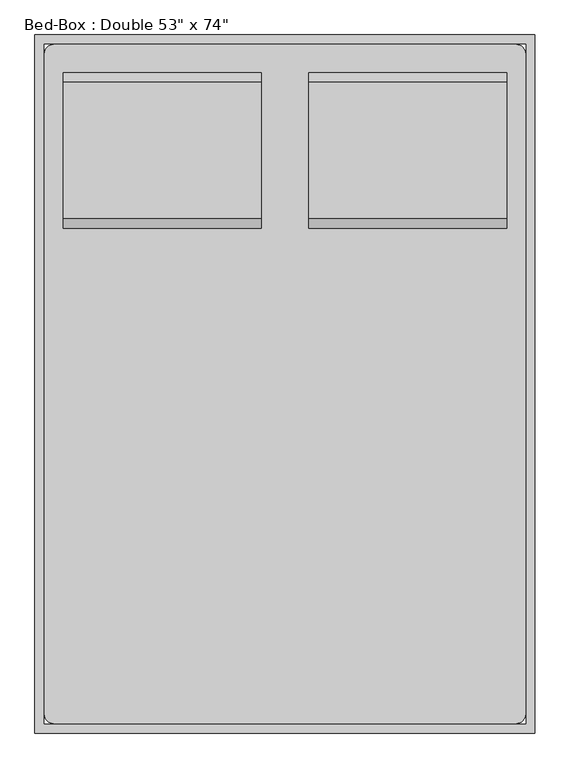
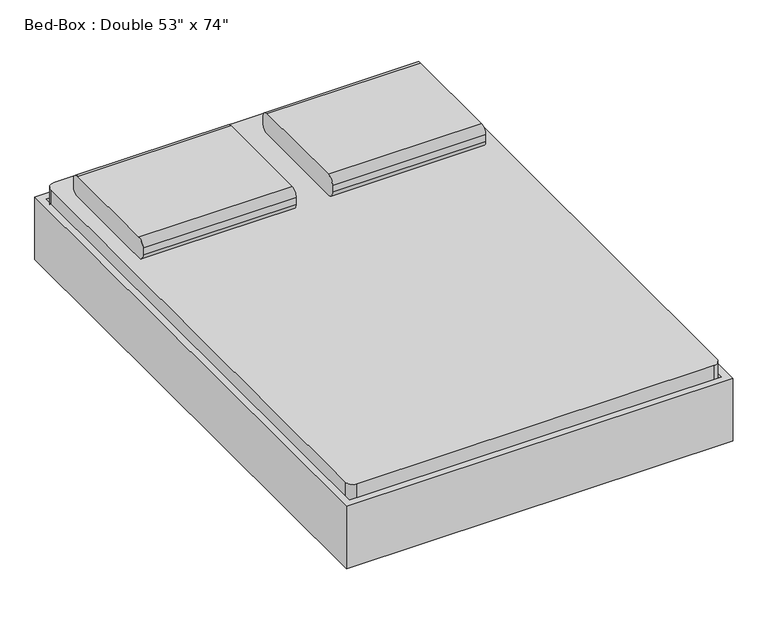
"""IFC4 building model written with IfcOpenShell, lengths in millimetres: furniture geometry."""

from ifc_helpers import new_model, si_unit, point, frame, frame_2d, origin, place, context, project, spatial, polyline, circle_curve, trimmed, segment, composite_curve, outline, extrude, source, transform, mapped, element, save
from ifc_brep_helpers import plane_surface, cylinder_surface, revolved_surface, advanced_brep


def furniture_b58f7881(model_context):
    return source(origin(), model_context, "Body", "SolidModel", [
        advanced_brep(
        [(-308.547541, -869.4295082, 196.85), (-308.547541, -869.4295082, 177.8), (-308.547541, -945.6295082, 177.8), (-308.547541, -945.6295082, 196.85), (-245.6113525, -869.4295082, 196.85), (-257.747541, -869.4295082, 177.8), (-257.747541, -945.6295082, 177.8), (-245.6113525, -945.6295082, 196.85), (-164.4115092, -869.4295082, 22.716374), (-181.6766725, -869.4295082, 14.6654962), (-181.6766725, -945.6295082, 14.6654962), (-164.4115092, -945.6295082, 22.716374), (-158.6564547, -869.4295082, 0.0), (-158.6564547, -869.4295082, 19.05), (-158.6564547, -945.6295082, 0.0), (-158.6564547, -945.6295082, 19.05), (-80.0439489, -869.4295082, 19.05), (-80.0439489, -869.4295082, 0.0), (-80.0439489, -945.6295082, 0.0), (-80.0439489, -945.6295082, 19.05), (-67.3439489, -869.4295082, 3.4029547), (-76.8689489, -869.4295082, 19.9007387), (-67.3439489, -945.6295082, 3.4029547), (-76.8689489, -945.6295082, 19.9007387), (-12.3513357, -869.4295082, 57.15), (-7.2469036, -869.4295082, 38.1), (-7.2469036, -945.6295082, 38.1), (-12.3513357, -945.6295082, 57.15), (690.6562537, -869.4295082, 57.15), (685.5518216, -869.4295082, 38.1), (685.5518216, -945.6295082, 38.1), (690.6562537, -945.6295082, 57.15), (755.1738669, -869.4295082, 19.9007387), (745.6488669, -869.4295082, 3.4029547), (745.6488669, -945.6295082, 3.4029547), (755.1738669, -945.6295082, 19.9007387), (758.3488669, -869.4295082, 0.0), (758.3488669, -869.4295082, 19.05), (758.3488669, -945.6295082, 0.0), (758.3488669, -945.6295082, 19.05), (836.9613728, -869.4295082, 19.05), (836.9613728, -869.4295082, 0.0), (836.9613728, -945.6295082, 0.0), (836.9613728, -945.6295082, 19.05), (859.9815906, -869.4295082, 14.6654962), (842.7164272, -869.4295082, 22.716374), (859.9815906, -945.6295082, 14.6654962), (842.7164272, -945.6295082, 22.716374), (923.9162705, -869.4295082, 196.85), (936.052459, -869.4295082, 177.8), (936.052459, -945.6295082, 177.8), (923.9162705, -945.6295082, 196.85), (986.852459, -869.4295082, 196.85), (986.852459, -945.6295082, 196.85), (986.852459, -945.6295082, 177.8), (986.852459, -869.4295082, 177.8)],
        [
            (0, 1),
            (1, 2),
            (2, 3),
            (3, 0),
            (0, 4),
            (4, 5),
            (5, 1),
            (5, 6),
            (6, 2),
            (6, 7),
            (7, 3),
            (7, 4),
            (4, 8),
            (8, 9),
            (9, 5),
            (9, 10),
            (10, 6),
            (10, 11),
            (11, 7),
            (11, 8),
            (12, 9, circle_curve(frame((-158.6564547, -869.4295082, 25.4), z_axis=(0.0, 1.0, 0.0), x_axis=(-0.906307787036663, 0.0, -0.4226182617406713)), 25.4)),
            (8, 13, circle_curve(frame((-158.6564547, -869.4295082, 25.4), z_axis=(0.0, -1.0, 0.0), x_axis=(-0.906307787036663, 0.0, -0.4226182617406713)), 6.35)),
            (13, 12),
            (14, 10, circle_curve(frame((-158.6564547, -945.6295082, 25.4), z_axis=(0.0, 1.0, 0.0), x_axis=(-0.906307787036663, 0.0, -0.4226182617406713)), 25.4)),
            (12, 14),
            (15, 11, circle_curve(frame((-158.6564547, -945.6295082, 25.4), z_axis=(0.0, 1.0, 0.0), x_axis=(-0.906307787036663, 0.0, -0.4226182617406713)), 6.35)),
            (14, 15),
            (15, 13),
            (13, 16),
            (16, 17),
            (17, 12),
            (17, 18),
            (18, 14),
            (18, 19),
            (19, 15),
            (19, 16),
            (20, 17, circle_curve(frame((-80.0439489, -869.4295082, 25.4), z_axis=(0.0, 1.0, 0.0), x_axis=(0.0, 0.0, -1.0)), 25.4)),
            (16, 21, circle_curve(frame((-80.0439489, -869.4295082, 25.4), z_axis=(0.0, -1.0, 0.0), x_axis=(0.0, 0.0, -1.0)), 6.35)),
            (21, 20),
            (22, 18, circle_curve(frame((-80.0439489, -945.6295082, 25.4), z_axis=(0.0, 1.0, 0.0), x_axis=(0.0, 0.0, -1.0)), 25.4)),
            (20, 22),
            (23, 19, circle_curve(frame((-80.0439489, -945.6295082, 25.4), z_axis=(0.0, 1.0, 0.0), x_axis=(0.0, 0.0, -1.0)), 6.35)),
            (22, 23),
            (23, 21),
            (21, 24),
            (24, 25),
            (25, 20),
            (25, 26),
            (26, 22),
            (26, 27),
            (27, 23),
            (27, 24),
            (24, 28),
            (28, 29),
            (29, 25),
            (29, 30),
            (30, 26),
            (30, 31),
            (31, 27),
            (31, 28),
            (28, 32),
            (32, 33),
            (33, 29),
            (33, 34),
            (34, 30),
            (34, 35),
            (35, 31),
            (35, 32),
            (36, 33, circle_curve(frame((758.3488669, -869.4295082, 25.4), z_axis=(0.0, 1.0, 0.0), x_axis=(-0.5000000000000479, 0.0, -0.866025403784411)), 25.4)),
            (32, 37, circle_curve(frame((758.3488669, -869.4295082, 25.4), z_axis=(0.0, -1.0, 0.0), x_axis=(-0.5000000000000479, 0.0, -0.866025403784411)), 6.35)),
            (37, 36),
            (38, 34, circle_curve(frame((758.3488669, -945.6295082, 25.4), z_axis=(0.0, 1.0, 0.0), x_axis=(-0.5000000000000479, 0.0, -0.866025403784411)), 25.4)),
            (36, 38),
            (39, 35, circle_curve(frame((758.3488669, -945.6295082, 25.4), z_axis=(0.0, 1.0, 0.0), x_axis=(-0.5000000000000479, 0.0, -0.866025403784411)), 6.35)),
            (38, 39),
            (39, 37),
            (37, 40),
            (40, 41),
            (41, 36),
            (41, 42),
            (42, 38),
            (42, 43),
            (43, 39),
            (43, 40),
            (44, 41, circle_curve(frame((836.9613728, -869.4295082, 25.4), z_axis=(0.0, 1.0, 0.0), x_axis=(0.0, 0.0, -1.0)), 25.4)),
            (40, 45, circle_curve(frame((836.9613728, -869.4295082, 25.4), z_axis=(0.0, -1.0, 0.0), x_axis=(0.0, 0.0, -1.0)), 6.35)),
            (45, 44),
            (46, 42, circle_curve(frame((836.9613728, -945.6295082, 25.4), z_axis=(0.0, 1.0, 0.0), x_axis=(0.0, 0.0, -1.0)), 25.4)),
            (44, 46),
            (47, 43, circle_curve(frame((836.9613728, -945.6295082, 25.4), z_axis=(0.0, 1.0, 0.0), x_axis=(0.0, 0.0, -1.0)), 6.35)),
            (46, 47),
            (47, 45),
            (45, 48),
            (48, 49),
            (49, 44),
            (49, 50),
            (50, 46),
            (50, 51),
            (51, 47),
            (51, 48),
            (52, 53),
            (53, 54),
            (54, 55),
            (55, 52),
            (48, 52),
            (55, 49),
            (54, 50),
            (53, 51),
        ],
        [
            plane_surface(frame((-308.547541, -1174.2295082, -127.5947323), z_axis=(-1.0, 0.0, 0.0), x_axis=(0.0, 1.0, 0.0))),
            plane_surface(frame((-308.547541, -869.4295082, 196.85), z_axis=(0.0, 1.0, 0.0), x_axis=(1.0, 0.0, 0.0))),
            plane_surface(frame((-308.547541, -869.4295082, 177.8), z_axis=(0.0, 0.0, -1.0), x_axis=(1.0, 0.0, 0.0))),
            plane_surface(frame((-308.547541, -945.6295082, 177.8), z_axis=(0.0, -1.0, 0.0), x_axis=(1.0, 0.0, 0.0))),
            plane_surface(frame((-308.547541, -945.6295082, 196.85), z_axis=(0.0, 0.0, 1.0), x_axis=(1.0, 0.0, 0.0))),
            plane_surface(frame((-245.6113525, -869.4295082, 196.85), z_axis=(0.0, 1.0, 0.0), x_axis=(0.422618261740671, 0.0, -0.9063077870366633))),
            plane_surface(frame((-257.747541, -869.4295082, 177.8), z_axis=(-0.9063077870366631, 0.0, -0.42261826174067113), x_axis=(0.42261826174067113, 0.0, -0.9063077870366631))),
            plane_surface(frame((-257.747541, -945.6295082, 177.8), z_axis=(0.0, -1.0, 0.0), x_axis=(0.42261826174067135, 0.0, -0.906307787036663))),
            plane_surface(frame((-245.6113525, -945.6295082, 196.85), z_axis=(0.9063077870366631, 0.0, 0.4226182617406713), x_axis=(0.4226182617406713, 0.0, -0.9063077870366631))),
            plane_surface(frame((-158.6564547, -869.4295082, 25.4), z_axis=(0.0, 1.0, 0.0), x_axis=(-0.906307787036663, 0.0, -0.4226182617406713))),
            cylinder_surface(frame((-158.6564547, -1174.2295082, 25.4), z_axis=(0.0, -1.0, 0.0), x_axis=(-0.906307787036663, 0.0, -0.4226182617406713)), 25.4),
            plane_surface(frame((-158.6564547, -945.6295082, 25.4), z_axis=(0.0, -1.0, 0.0), x_axis=(-0.906307787036663, 0.0, -0.4226182617406713))),
            revolved_surface(polyline([(-164.41150914768284, -945.6295082, 22.716374037946736), (-164.41150914768284, -869.4295082, 22.716374037946736)]), (-158.6564547, -1174.2295082, 25.4), (0.0, -1.0, 0.0)),
            plane_surface(frame((-158.6564547, -869.4295082, 19.05), z_axis=(0.0, 1.0, 0.0), x_axis=(1.0, 0.0, 0.0))),
            plane_surface(frame((-158.6564547, -869.4295082, 0.0), z_axis=(0.0, 0.0, -1.0), x_axis=(1.0, 0.0, 0.0))),
            plane_surface(frame((-158.6564547, -945.6295082, 0.0), z_axis=(0.0, -1.0, 0.0), x_axis=(1.0, 0.0, 0.0))),
            plane_surface(frame((-158.6564547, -945.6295082, 19.05), z_axis=(0.0, 0.0, 1.0), x_axis=(1.0, 0.0, 0.0))),
            plane_surface(frame((-80.0439489, -869.4295082, 25.4), z_axis=(0.0, 1.0, 0.0), x_axis=(0.0, 0.0, -1.0))),
            cylinder_surface(frame((-80.0439489, -1174.2295082, 25.4), z_axis=(0.0, -1.0, 0.0), x_axis=(0.0, 0.0, -1.0)), 25.4),
            plane_surface(frame((-80.0439489, -945.6295082, 25.4), z_axis=(0.0, -1.0, 0.0), x_axis=(0.0, 0.0, -1.0))),
            revolved_surface(polyline([(-80.0439489, -945.6295082, 19.049999999999997), (-80.0439489, -869.4295082, 19.049999999999997)]), (-80.0439489, -1174.2295082, 25.4), (0.0, -1.0, 0.0)),
            plane_surface(frame((-76.8689489, -869.4295082, 19.9007387), z_axis=(0.0, 1.0, 0.0), x_axis=(0.8660254037844785, 0.0, 0.499999999999931))),
            plane_surface(frame((-67.3439489, -869.4295082, 3.4029547), z_axis=(0.499999999999931, 0.0, -0.8660254037844785), x_axis=(0.8660254037844785, 0.0, 0.499999999999931))),
            plane_surface(frame((-67.3439489, -945.6295082, 3.4029547), z_axis=(0.0, -1.0, 0.0), x_axis=(0.8660254037844786, 0.0, 0.49999999999993094))),
            plane_surface(frame((-76.8689489, -945.6295082, 19.9007387), z_axis=(-0.4999999999999312, 0.0, 0.8660254037844785), x_axis=(0.8660254037844785, 0.0, 0.4999999999999312))),
            plane_surface(frame((-12.3513357, -869.4295082, 57.15), z_axis=(0.0, 1.0, 0.0), x_axis=(1.0, 0.0, 0.0))),
            plane_surface(frame((-7.2469036, -869.4295082, 38.1), z_axis=(0.0, 0.0, -1.0), x_axis=(1.0, 0.0, 0.0))),
            plane_surface(frame((-7.2469036, -945.6295082, 38.1), z_axis=(0.0, -1.0, 0.0), x_axis=(1.0, 0.0, 0.0))),
            plane_surface(frame((-12.3513357, -945.6295082, 57.15), z_axis=(0.0, 0.0, 1.0), x_axis=(1.0, 0.0, 0.0))),
            plane_surface(frame((690.6562537, -869.4295082, 57.15), z_axis=(0.0, 1.0, 0.0), x_axis=(0.8660254037844091, 0.0, -0.5000000000000514))),
            plane_surface(frame((685.5518216, -869.4295082, 38.1), z_axis=(-0.5000000000000502, 0.0, -0.8660254037844097), x_axis=(0.8660254037844097, 0.0, -0.5000000000000502))),
            plane_surface(frame((685.5518216, -945.6295082, 38.1), z_axis=(0.0, -1.0, 0.0), x_axis=(0.86602540378441, 0.0, -0.5000000000000498))),
            plane_surface(frame((690.6562537, -945.6295082, 57.15), z_axis=(0.5000000000000505, 0.0, 0.8660254037844095), x_axis=(0.8660254037844095, 0.0, -0.5000000000000505))),
            plane_surface(frame((758.3488669, -869.4295082, 25.4), z_axis=(0.0, 1.0000000000000002, 0.0), x_axis=(-0.500000000000048, 0.0, -0.8660254037844111))),
            cylinder_surface(frame((758.3488669, -1174.2295082, 25.4), z_axis=(0.0, -1.0, 0.0), x_axis=(-0.5000000000000479, 0.0, -0.866025403784411)), 25.4),
            plane_surface(frame((758.3488669, -945.6295082, 25.4), z_axis=(0.0, -1.0000000000000002, 0.0), x_axis=(-0.500000000000048, 0.0, -0.8660254037844111))),
            revolved_surface(polyline([(755.1738668999997, -945.6295082, 19.90073868596899), (755.1738668999997, -869.4295082, 19.90073868596899)]), (758.3488669, -1174.2295082, 25.4), (0.0, -1.0, 0.0)),
            plane_surface(frame((758.3488669, -869.4295082, 19.05), z_axis=(0.0, 1.0, 0.0), x_axis=(1.0, 0.0, 0.0))),
            plane_surface(frame((758.3488669, -869.4295082, 0.0), z_axis=(0.0, 0.0, -1.0), x_axis=(1.0, 0.0, 0.0))),
            plane_surface(frame((758.3488669, -945.6295082, 0.0), z_axis=(0.0, -1.0, 0.0), x_axis=(1.0, 0.0, 0.0))),
            plane_surface(frame((758.3488669, -945.6295082, 19.05), z_axis=(0.0, 0.0, 1.0), x_axis=(1.0, 0.0, 0.0))),
            plane_surface(frame((836.9613728, -869.4295082, 25.4), z_axis=(0.0, 1.0, 0.0), x_axis=(0.0, 0.0, -1.0))),
            cylinder_surface(frame((836.9613728, -1174.2295082, 25.4), z_axis=(0.0, -1.0, 0.0), x_axis=(0.0, 0.0, -1.0)), 25.4),
            plane_surface(frame((836.9613728, -945.6295082, 25.4), z_axis=(0.0, -1.0, 0.0), x_axis=(0.0, 0.0, -1.0))),
            revolved_surface(polyline([(836.9613728, -945.6295082, 19.049999999999997), (836.9613728, -869.4295082, 19.049999999999997)]), (836.9613728, -1174.2295082, 25.4), (0.0, -1.0, 0.0)),
            plane_surface(frame((842.7164272, -869.4295082, 22.716374), z_axis=(0.0, 1.0, 0.0), x_axis=(0.4226182617405411, 0.0, 0.9063077870367238))),
            plane_surface(frame((859.9815906, -869.4295082, 14.6654962), z_axis=(0.9063077870367237, 0.0, -0.42261826174054157), x_axis=(0.42261826174054157, 0.0, 0.9063077870367237))),
            plane_surface(frame((859.9815906, -945.6295082, 14.6654962), z_axis=(0.0, -1.0, 0.0), x_axis=(0.4226182617405412, 0.0, 0.9063077870367238))),
            plane_surface(frame((842.7164272, -945.6295082, 22.716374), z_axis=(-0.906307787036724, 0.0, 0.422618261740541), x_axis=(0.422618261740541, 0.0, 0.906307787036724))),
            plane_surface(frame((986.852459, -1174.2295082, -127.5947323), z_axis=(1.0, 0.0, 0.0), x_axis=(0.0, 1.0, 0.0))),
            plane_surface(frame((923.9162705, -869.4295082, 196.85), z_axis=(0.0, 1.0, 0.0), x_axis=(1.0, 0.0, 0.0))),
            plane_surface(frame((936.052459, -869.4295082, 177.8), z_axis=(0.0, 0.0, -1.0), x_axis=(1.0, 0.0, 0.0))),
            plane_surface(frame((936.052459, -945.6295082, 177.8), z_axis=(0.0, -1.0, 0.0), x_axis=(1.0, 0.0, 0.0))),
            plane_surface(frame((923.9162705, -945.6295082, 196.85), z_axis=(0.0, 0.0, 1.0), x_axis=(1.0, 0.0, 0.0))),
        ],
        [
            (0, [[1, 2, 3, 4]]),
            (1, [[-1, 5, 6, 7]]),
            (2, [[-2, -7, 8, 9]]),
            (3, [[-3, -9, 10, 11]]),
            (4, [[-4, -11, 12, -5]]),
            (5, [[-6, 13, 14, 15]]),
            (6, [[-8, -15, 16, 17]]),
            (7, [[-10, -17, 18, 19]]),
            (8, [[-12, -19, 20, -13]]),
            (9, [[21, -14, 22, 23]]),
            (10, [[24, -16, -21, 25]]),
            (11, [[26, -18, -24, 27]]),
            (12, [[-22, -20, -26, 28]]),
            (13, [[-23, 29, 30, 31]]),
            (14, [[-25, -31, 32, 33]]),
            (15, [[-27, -33, 34, 35]]),
            (16, [[-28, -35, 36, -29]]),
            (17, [[37, -30, 38, 39]]),
            (18, [[40, -32, -37, 41]]),
            (19, [[42, -34, -40, 43]]),
            (20, [[-38, -36, -42, 44]]),
            (21, [[-39, 45, 46, 47]]),
            (22, [[-41, -47, 48, 49]]),
            (23, [[-43, -49, 50, 51]]),
            (24, [[-44, -51, 52, -45]]),
            (25, [[-46, 53, 54, 55]]),
            (26, [[-48, -55, 56, 57]]),
            (27, [[-50, -57, 58, 59]]),
            (28, [[-52, -59, 60, -53]]),
            (29, [[-54, 61, 62, 63]]),
            (30, [[-56, -63, 64, 65]]),
            (31, [[-58, -65, 66, 67]]),
            (32, [[-60, -67, 68, -61]]),
            (33, [[69, -62, 70, 71]]),
            (34, [[72, -64, -69, 73]]),
            (35, [[74, -66, -72, 75]]),
            (36, [[-70, -68, -74, 76]]),
            (37, [[-71, 77, 78, 79]]),
            (38, [[-73, -79, 80, 81]]),
            (39, [[-75, -81, 82, 83]]),
            (40, [[-76, -83, 84, -77]]),
            (41, [[85, -78, 86, 87]]),
            (42, [[88, -80, -85, 89]]),
            (43, [[90, -82, -88, 91]]),
            (44, [[-86, -84, -90, 92]]),
            (45, [[-87, 93, 94, 95]]),
            (46, [[-89, -95, 96, 97]]),
            (47, [[-91, -97, 98, 99]]),
            (48, [[-92, -99, 100, -93]]),
            (49, [[101, 102, 103, 104]]),
            (50, [[-94, 105, -104, 106]]),
            (51, [[-96, -106, -103, 107]]),
            (52, [[-98, -107, -102, 108]]),
            (53, [[-100, -108, -101, -105]]),
        ],
    ),
        extrude(outline(composite_curve([segment(polyline([(-283.147541, 679.9704918), (961.452459, 679.9704918)]), True, "CONTINUOUS"), segment(trimmed(circle_curve(frame_2d((961.452459, 654.5704918)), 25.4), [point((961.452459, 679.9704918))], [point((986.852459, 654.5704918))], False, "CARTESIAN"), True, "CONTINUOUS"), segment(polyline([(986.852459, 654.5704918), (986.852459, -1123.4295082)]), True, "CONTINUOUS"), segment(trimmed(circle_curve(frame_2d((961.452459, -1123.4295082)), 25.4), [point((986.852459, -1123.4295082))], [point((961.452459, -1148.8295082))], False, "CARTESIAN"), True, "CONTINUOUS"), segment(polyline([(961.452459, -1148.8295082), (-283.147541, -1148.8295082)]), True, "CONTINUOUS"), segment(trimmed(circle_curve(frame_2d((-283.147541, -1123.4295082)), 25.4), [point((-283.147541, -1148.8295082))], [point((-308.547541, -1123.4295082))], False, "CARTESIAN"), True, "CONTINUOUS"), segment(polyline([(-308.547541, -1123.4295082), (-308.547541, 654.5704918)]), True, "CONTINUOUS"), segment(trimmed(circle_curve(frame_2d((-283.147541, 654.5704918)), 25.4), [point((-308.547541, 654.5704918))], [point((-283.147541, 679.9704918))], False, "CARTESIAN"), True, "CONTINUOUS")], self_intersect=False)), frame((0.0, 0.0, 203.2), z_axis=(0.0, 0.0, 1.0), x_axis=(1.0, 0.0, 0.0)), (0.0, 0.0, 1.0), 203.2),
        advanced_brep(
        [(-308.2231784, 451.3704918, 177.8), (-308.2231784, 375.1704918, 177.8), (-308.2231784, 375.1704918, 196.85), (-308.2231784, 451.3704918, 196.85), (-257.4231784, 451.3704918, 177.8), (-257.4231784, 375.1704918, 177.8), (-245.2869899, 375.1704918, 196.85), (-245.2869899, 451.3704918, 196.85), (-181.3523099, 451.3704918, 14.6654962), (-181.3523099, 375.1704918, 14.6654962), (-164.0871466, 375.1704918, 22.716374), (-164.0871466, 451.3704918, 22.716374), (-158.3320921, 375.1704918, 0.0), (-158.3320921, 451.3704918, 0.0), (-158.3320921, 375.1704918, 19.05), (-158.3320921, 451.3704918, 19.05), (-79.7195862, 451.3704918, 0.0), (-79.7195862, 375.1704918, 0.0), (-79.7195862, 375.1704918, 19.05), (-79.7195862, 451.3704918, 19.05), (-67.0195862, 375.1704918, 3.4029547), (-67.0195862, 451.3704918, 3.4029547), (-76.5445862, 375.1704918, 19.9007387), (-76.5445862, 451.3704918, 19.9007387), (-6.922541, 451.3704918, 38.1), (-6.922541, 375.1704918, 38.1), (-12.0269731, 375.1704918, 57.15), (-12.0269731, 451.3704918, 57.15), (685.5518216, 451.3704918, 38.1), (685.5518216, 375.1704918, 38.1), (690.6562537, 375.1704918, 57.15), (690.6562537, 451.3704918, 57.15), (745.6488669, 451.3704918, 3.4029547), (745.6488669, 375.1704918, 3.4029547), (755.1738669, 375.1704918, 19.9007387), (755.1738669, 451.3704918, 19.9007387), (758.3488669, 375.1704918, 0.0), (758.3488669, 451.3704918, 0.0), (758.3488669, 375.1704918, 19.05), (758.3488669, 451.3704918, 19.05), (836.9613728, 451.3704918, 0.0), (836.9613728, 375.1704918, 0.0), (836.9613728, 375.1704918, 19.05), (836.9613728, 451.3704918, 19.05), (859.9815906, 375.1704918, 14.6654962), (859.9815906, 451.3704918, 14.6654962), (842.7164272, 375.1704918, 22.716374), (842.7164272, 451.3704918, 22.716374), (936.052459, 451.3704918, 177.8), (936.052459, 375.1704918, 177.8), (923.9162705, 375.1704918, 196.85), (923.9162705, 451.3704918, 196.85), (986.852459, 451.3704918, 177.8), (986.852459, 451.3704918, 196.85), (986.852459, 375.1704918, 196.85), (986.852459, 375.1704918, 177.8)],
        [
            (0, 1),
            (1, 2),
            (2, 3),
            (3, 0),
            (0, 4),
            (4, 5),
            (5, 1),
            (5, 6),
            (6, 2),
            (6, 7),
            (7, 3),
            (7, 4),
            (4, 8),
            (8, 9),
            (9, 5),
            (9, 10),
            (10, 6),
            (10, 11),
            (11, 7),
            (11, 8),
            (12, 9, circle_curve(frame((-158.3320921, 375.1704918, 25.4), z_axis=(0.0, 1.0, 0.0), x_axis=(-0.9063077870366486, 0.0, -0.42261826174070233)), 25.4)),
            (8, 13, circle_curve(frame((-158.3320921, 451.3704918, 25.4), z_axis=(0.0, -1.0, 0.0), x_axis=(-0.9063077870366486, 0.0, -0.42261826174070233)), 25.4)),
            (13, 12),
            (14, 10, circle_curve(frame((-158.3320921, 375.1704918, 25.4), z_axis=(0.0, 1.0, 0.0), x_axis=(-0.9063077870366486, 0.0, -0.42261826174070233)), 6.35)),
            (12, 14),
            (15, 11, circle_curve(frame((-158.3320921, 451.3704918, 25.4), z_axis=(0.0, 1.0, 0.0), x_axis=(-0.9063077870366486, 0.0, -0.42261826174070233)), 6.35)),
            (14, 15),
            (15, 13),
            (13, 16),
            (16, 17),
            (17, 12),
            (17, 18),
            (18, 14),
            (18, 19),
            (19, 15),
            (19, 16),
            (20, 17, circle_curve(frame((-79.7195862, 375.1704918, 25.4), z_axis=(0.0, 1.0, 0.0), x_axis=(0.0, 0.0, -1.0)), 25.4)),
            (16, 21, circle_curve(frame((-79.7195862, 451.3704918, 25.4), z_axis=(0.0, -1.0, 0.0), x_axis=(0.0, 0.0, -1.0)), 25.4)),
            (21, 20),
            (22, 18, circle_curve(frame((-79.7195862, 375.1704918, 25.4), z_axis=(0.0, 1.0, 0.0), x_axis=(0.0, 0.0, -1.0)), 6.35)),
            (20, 22),
            (23, 19, circle_curve(frame((-79.7195862, 451.3704918, 25.4), z_axis=(0.0, 1.0, 0.0), x_axis=(0.0, 0.0, -1.0)), 6.35)),
            (22, 23),
            (23, 21),
            (21, 24),
            (24, 25),
            (25, 20),
            (25, 26),
            (26, 22),
            (26, 27),
            (27, 23),
            (27, 24),
            (24, 28),
            (28, 29),
            (29, 25),
            (29, 30),
            (30, 26),
            (30, 31),
            (31, 27),
            (31, 28),
            (28, 32),
            (32, 33),
            (33, 29),
            (33, 34),
            (34, 30),
            (34, 35),
            (35, 31),
            (35, 32),
            (36, 33, circle_curve(frame((758.3488669, 375.1704918, 25.4), z_axis=(0.0, 1.0, 0.0), x_axis=(-0.5000000000000463, 0.0, -0.8660254037844118)), 25.4)),
            (32, 37, circle_curve(frame((758.3488669, 451.3704918, 25.4), z_axis=(0.0, -1.0, 0.0), x_axis=(-0.5000000000000463, 0.0, -0.8660254037844118)), 25.4)),
            (37, 36),
            (38, 34, circle_curve(frame((758.3488669, 375.1704918, 25.4), z_axis=(0.0, 1.0, 0.0), x_axis=(-0.5000000000000463, 0.0, -0.8660254037844118)), 6.35)),
            (36, 38),
            (39, 35, circle_curve(frame((758.3488669, 451.3704918, 25.4), z_axis=(0.0, 1.0, 0.0), x_axis=(-0.5000000000000463, 0.0, -0.8660254037844118)), 6.35)),
            (38, 39),
            (39, 37),
            (37, 40),
            (40, 41),
            (41, 36),
            (41, 42),
            (42, 38),
            (42, 43),
            (43, 39),
            (43, 40),
            (44, 41, circle_curve(frame((836.9613728, 375.1704918, 25.4), z_axis=(0.0, 1.0, 0.0), x_axis=(0.0, 0.0, -1.0)), 25.4)),
            (40, 45, circle_curve(frame((836.9613728, 451.3704918, 25.4), z_axis=(0.0, -1.0, 0.0), x_axis=(0.0, 0.0, -1.0)), 25.4)),
            (45, 44),
            (46, 42, circle_curve(frame((836.9613728, 375.1704918, 25.4), z_axis=(0.0, 1.0, 0.0), x_axis=(0.0, 0.0, -1.0)), 6.35)),
            (44, 46),
            (47, 43, circle_curve(frame((836.9613728, 451.3704918, 25.4), z_axis=(0.0, 1.0, 0.0), x_axis=(0.0, 0.0, -1.0)), 6.35)),
            (46, 47),
            (47, 45),
            (45, 48),
            (48, 49),
            (49, 44),
            (49, 50),
            (50, 46),
            (50, 51),
            (51, 47),
            (51, 48),
            (52, 53),
            (53, 54),
            (54, 55),
            (55, 52),
            (48, 52),
            (55, 49),
            (54, 50),
            (53, 51),
        ],
        [
            plane_surface(frame((-308.2231784, 705.3704918, -152.9490627), z_axis=(-1.0, 0.0, 0.0), x_axis=(0.0, 1.0, 0.0))),
            plane_surface(frame((-308.2231784, 451.3704918, 177.8), z_axis=(0.0, 0.0, -1.0), x_axis=(1.0, 0.0, 0.0))),
            plane_surface(frame((-308.2231784, 375.1704918, 177.8), z_axis=(0.0, -1.0, 0.0), x_axis=(1.0, 0.0, 0.0))),
            plane_surface(frame((-308.2231784, 375.1704918, 196.85), z_axis=(0.0, 0.0, 1.0), x_axis=(1.0, 0.0, 0.0))),
            plane_surface(frame((-308.2231784, 451.3704918, 196.85), z_axis=(0.0, 1.0, 0.0), x_axis=(1.0, 0.0, 0.0))),
            plane_surface(frame((-257.4231784, 451.3704918, 177.8), z_axis=(-0.9063077870366488, 0.0, -0.42261826174070194), x_axis=(0.42261826174070194, 0.0, -0.9063077870366488))),
            plane_surface(frame((-257.4231784, 375.1704918, 177.8), z_axis=(0.0, -1.0, 0.0), x_axis=(0.42261826174070194, 0.0, -0.9063077870366488))),
            plane_surface(frame((-245.2869899, 375.1704918, 196.85), z_axis=(0.9063077870366487, 0.0, 0.4226182617407021), x_axis=(0.4226182617407021, 0.0, -0.9063077870366487))),
            plane_surface(frame((-245.2869899, 451.3704918, 196.85), z_axis=(0.0, 1.0, 0.0), x_axis=(0.4226182617407021, 0.0, -0.9063077870366487))),
            cylinder_surface(frame((-158.3320921, 705.3704918, 25.4), z_axis=(0.0, -1.0, 0.0), x_axis=(-0.9063077870366486, 0.0, -0.42261826174070233)), 25.4),
            plane_surface(frame((-158.3320921, 375.1704918, 25.4), z_axis=(0.0, -1.0, 0.0), x_axis=(-0.9063077870366486, 0.0, -0.42261826174070233))),
            revolved_surface(polyline([(-164.08714654768272, 375.1704918, 22.71637403794654), (-164.08714654768272, 451.3704918, 22.71637403794654)]), (-158.3320921, 705.3704918, 25.4), (0.0, -1.0, 0.0)),
            plane_surface(frame((-158.3320921, 451.3704918, 25.4), z_axis=(0.0, 1.0, 0.0), x_axis=(-0.9063077870366486, 0.0, -0.42261826174070233))),
            plane_surface(frame((-158.3320921, 451.3704918, 0.0), z_axis=(0.0, 0.0, -1.0), x_axis=(1.0, 0.0, 0.0))),
            plane_surface(frame((-158.3320921, 375.1704918, 0.0), z_axis=(0.0, -1.0, 0.0), x_axis=(1.0, 0.0, 0.0))),
            plane_surface(frame((-158.3320921, 375.1704918, 19.05), z_axis=(0.0, 0.0, 1.0), x_axis=(1.0, 0.0, 0.0))),
            plane_surface(frame((-158.3320921, 451.3704918, 19.05), z_axis=(0.0, 1.0, 0.0), x_axis=(1.0, 0.0, 0.0))),
            cylinder_surface(frame((-79.7195862, 705.3704918, 25.4), z_axis=(0.0, -1.0, 0.0), x_axis=(0.0, 0.0, -1.0)), 25.4),
            plane_surface(frame((-79.7195862, 375.1704918, 25.4), z_axis=(0.0, -1.0, 0.0), x_axis=(0.0, 0.0, -1.0))),
            revolved_surface(polyline([(-79.7195862, 375.1704918, 19.049999999999997), (-79.7195862, 451.3704918, 19.049999999999997)]), (-79.7195862, 705.3704918, 25.4), (0.0, -1.0, 0.0)),
            plane_surface(frame((-79.7195862, 451.3704918, 25.4), z_axis=(0.0, 1.0, 0.0), x_axis=(0.0, 0.0, -1.0))),
            plane_surface(frame((-67.0195862, 451.3704918, 3.4029547), z_axis=(0.4999999999998775, 0.0, -0.8660254037845094), x_axis=(0.8660254037845094, 0.0, 0.4999999999998775))),
            plane_surface(frame((-67.0195862, 375.1704918, 3.4029547), z_axis=(0.0, -1.0, 0.0), x_axis=(0.866025403784509, 0.0, 0.49999999999987826))),
            plane_surface(frame((-76.5445862, 375.1704918, 19.9007387), z_axis=(-0.49999999999987754, 0.0, 0.8660254037845093), x_axis=(0.8660254037845093, 0.0, 0.49999999999987754))),
            plane_surface(frame((-76.5445862, 451.3704918, 19.9007387), z_axis=(0.0, 1.0000000000000002, 0.0), x_axis=(0.8660254037845091, 0.0, 0.49999999999987815))),
            plane_surface(frame((-6.922541, 451.3704918, 38.1), z_axis=(0.0, 0.0, -1.0), x_axis=(1.0, 0.0, 0.0))),
            plane_surface(frame((-6.922541, 375.1704918, 38.1), z_axis=(0.0, -1.0, 0.0), x_axis=(1.0, 0.0, 0.0))),
            plane_surface(frame((-12.0269731, 375.1704918, 57.15), z_axis=(0.0, 0.0, 1.0), x_axis=(1.0, 0.0, 0.0))),
            plane_surface(frame((-12.0269731, 451.3704918, 57.15), z_axis=(0.0, 1.0, 0.0), x_axis=(1.0, 0.0, 0.0))),
            plane_surface(frame((685.5518216, 451.3704918, 38.1), z_axis=(-0.500000000000047, 0.0, -0.8660254037844116), x_axis=(0.8660254037844116, 0.0, -0.500000000000047))),
            plane_surface(frame((685.5518216, 375.1704918, 38.1), z_axis=(0.0, -1.0, 0.0), x_axis=(0.8660254037844122, 0.0, -0.5000000000000459))),
            plane_surface(frame((690.6562537, 375.1704918, 57.15), z_axis=(0.5000000000000461, 0.0, 0.8660254037844121), x_axis=(0.8660254037844121, 0.0, -0.5000000000000461))),
            plane_surface(frame((690.6562537, 451.3704918, 57.15), z_axis=(0.0, 1.0, 0.0), x_axis=(0.8660254037844127, 0.0, -0.500000000000045))),
            cylinder_surface(frame((758.3488669, 705.3704918, 25.4), z_axis=(0.0, -1.0, 0.0), x_axis=(-0.5000000000000463, 0.0, -0.8660254037844118)), 25.4),
            plane_surface(frame((758.3488669, 375.1704918, 25.4), z_axis=(0.0, -1.0000000000000002, 0.0), x_axis=(-0.5000000000000464, 0.0, -0.866025403784412))),
            revolved_surface(polyline([(755.1738668999997, 375.1704918, 19.90073868596898), (755.1738668999997, 451.3704918, 19.90073868596898)]), (758.3488669, 705.3704918, 25.4), (0.0, -1.0, 0.0)),
            plane_surface(frame((758.3488669, 451.3704918, 25.4), z_axis=(0.0, 1.0000000000000002, 0.0), x_axis=(-0.5000000000000464, 0.0, -0.866025403784412))),
            plane_surface(frame((758.3488669, 451.3704918, 0.0), z_axis=(0.0, 0.0, -1.0), x_axis=(1.0, 0.0, 0.0))),
            plane_surface(frame((758.3488669, 375.1704918, 0.0), z_axis=(0.0, -1.0, 0.0), x_axis=(1.0, 0.0, 0.0))),
            plane_surface(frame((758.3488669, 375.1704918, 19.05), z_axis=(0.0, 0.0, 1.0), x_axis=(1.0, 0.0, 0.0))),
            plane_surface(frame((758.3488669, 451.3704918, 19.05), z_axis=(0.0, 1.0, 0.0), x_axis=(1.0, 0.0, 0.0))),
            cylinder_surface(frame((836.9613728, 705.3704918, 25.4), z_axis=(0.0, -1.0, 0.0), x_axis=(0.0, 0.0, -1.0)), 25.4),
            plane_surface(frame((836.9613728, 375.1704918, 25.4), z_axis=(0.0, -1.0, 0.0), x_axis=(0.0, 0.0, -1.0))),
            revolved_surface(polyline([(836.9613728, 375.1704918, 19.049999999999997), (836.9613728, 451.3704918, 19.049999999999997)]), (836.9613728, 705.3704918, 25.4), (0.0, -1.0, 0.0)),
            plane_surface(frame((836.9613728, 451.3704918, 25.4), z_axis=(0.0, 1.0, 0.0), x_axis=(0.0, 0.0, -1.0))),
            plane_surface(frame((859.9815906, 451.3704918, 14.6654962), z_axis=(0.9063077870366797, 0.0, -0.42261826174063566), x_axis=(0.42261826174063566, 0.0, 0.9063077870366797))),
            plane_surface(frame((859.9815906, 375.1704918, 14.6654962), z_axis=(0.0, -1.0000000000000002, 0.0), x_axis=(0.4226182617406349, 0.0, 0.9063077870366801))),
            plane_surface(frame((842.7164272, 375.1704918, 22.716374), z_axis=(-0.9063077870366799, 0.0, 0.4226182617406354), x_axis=(0.4226182617406354, 0.0, 0.9063077870366799))),
            plane_surface(frame((842.7164272, 451.3704918, 22.716374), z_axis=(0.0, 1.0, 0.0), x_axis=(0.42261826174063555, 0.0, 0.9063077870366798))),
            plane_surface(frame((986.852459, 705.3704918, -152.9490627), z_axis=(1.0, 0.0, 0.0), x_axis=(0.0, 1.0, 0.0))),
            plane_surface(frame((936.052459, 451.3704918, 177.8), z_axis=(0.0, 0.0, -1.0), x_axis=(1.0, 0.0, 0.0))),
            plane_surface(frame((936.052459, 375.1704918, 177.8), z_axis=(0.0, -1.0, 0.0), x_axis=(1.0, 0.0, 0.0))),
            plane_surface(frame((923.9162705, 375.1704918, 196.85), z_axis=(0.0, 0.0, 1.0), x_axis=(1.0, 0.0, 0.0))),
            plane_surface(frame((923.9162705, 451.3704918, 196.85), z_axis=(0.0, 1.0, 0.0), x_axis=(1.0, 0.0, 0.0))),
        ],
        [
            (0, [[1, 2, 3, 4]]),
            (1, [[-1, 5, 6, 7]]),
            (2, [[-2, -7, 8, 9]]),
            (3, [[-3, -9, 10, 11]]),
            (4, [[-4, -11, 12, -5]]),
            (5, [[-6, 13, 14, 15]]),
            (6, [[-8, -15, 16, 17]]),
            (7, [[-10, -17, 18, 19]]),
            (8, [[-12, -19, 20, -13]]),
            (9, [[21, -14, 22, 23]]),
            (10, [[24, -16, -21, 25]]),
            (11, [[26, -18, -24, 27]]),
            (12, [[-22, -20, -26, 28]]),
            (13, [[-23, 29, 30, 31]]),
            (14, [[-25, -31, 32, 33]]),
            (15, [[-27, -33, 34, 35]]),
            (16, [[-28, -35, 36, -29]]),
            (17, [[37, -30, 38, 39]]),
            (18, [[40, -32, -37, 41]]),
            (19, [[42, -34, -40, 43]]),
            (20, [[-38, -36, -42, 44]]),
            (21, [[-39, 45, 46, 47]]),
            (22, [[-41, -47, 48, 49]]),
            (23, [[-43, -49, 50, 51]]),
            (24, [[-44, -51, 52, -45]]),
            (25, [[-46, 53, 54, 55]]),
            (26, [[-48, -55, 56, 57]]),
            (27, [[-50, -57, 58, 59]]),
            (28, [[-52, -59, 60, -53]]),
            (29, [[-54, 61, 62, 63]]),
            (30, [[-56, -63, 64, 65]]),
            (31, [[-58, -65, 66, 67]]),
            (32, [[-60, -67, 68, -61]]),
            (33, [[69, -62, 70, 71]]),
            (34, [[72, -64, -69, 73]]),
            (35, [[74, -66, -72, 75]]),
            (36, [[-70, -68, -74, 76]]),
            (37, [[-71, 77, 78, 79]]),
            (38, [[-73, -79, 80, 81]]),
            (39, [[-75, -81, 82, 83]]),
            (40, [[-76, -83, 84, -77]]),
            (41, [[85, -78, 86, 87]]),
            (42, [[88, -80, -85, 89]]),
            (43, [[90, -82, -88, 91]]),
            (44, [[-86, -84, -90, 92]]),
            (45, [[-87, 93, 94, 95]]),
            (46, [[-89, -95, 96, 97]]),
            (47, [[-91, -97, 98, 99]]),
            (48, [[-92, -99, 100, -93]]),
            (49, [[101, 102, 103, 104]]),
            (50, [[-94, 105, -104, 106]]),
            (51, [[-96, -106, -103, 107]]),
            (52, [[-98, -107, -102, 108]]),
            (53, [[-100, -108, -101, -105]]),
        ],
    ),
        extrude(outline(composite_curve([segment(polyline([(578.3704918, 406.4), (210.0704918, 406.4)]), True, "CONTINUOUS"), segment(trimmed(circle_curve(frame_2d((210.0704918, 431.8)), 25.4), [point((210.0704918, 406.4))], [point((184.6704918, 431.8))], False, "CARTESIAN"), True, "CONTINUOUS"), segment(polyline([(184.6704918, 431.8), (184.6704918, 457.2)]), True, "CONTINUOUS"), segment(trimmed(circle_curve(frame_2d((210.0704918, 457.2)), 25.4), [point((184.6704918, 457.2))], [point((210.0704918, 482.6))], False, "CARTESIAN"), True, "CONTINUOUS"), segment(polyline([(210.0704918, 482.6), (578.3704918, 482.6)]), True, "CONTINUOUS"), segment(trimmed(circle_curve(frame_2d((578.3704918, 457.2)), 25.4), [point((578.3704918, 482.6))], [point((603.7704918, 457.2))], False, "CARTESIAN"), True, "CONTINUOUS"), segment(polyline([(603.7704918, 457.2), (603.7704918, 431.8)]), True, "CONTINUOUS"), segment(trimmed(circle_curve(frame_2d((578.3704918, 431.8)), 25.4), [point((603.7704918, 431.8))], [point((578.3704918, 406.4))], False, "CARTESIAN"), True, "CONTINUOUS")], self_intersect=False)), frame((-257.747541, 0.0, 0.0), z_axis=(1.0, 0.0, 0.0), x_axis=(0.0, 1.0, 0.0)), (0.0, 0.0, 1.0), 533.4),
        extrude(outline(composite_curve([segment(polyline([(578.3704918, 406.4), (210.0704918, 406.4)]), True, "CONTINUOUS"), segment(trimmed(circle_curve(frame_2d((210.0704918, 431.8)), 25.4), [point((210.0704918, 406.4))], [point((184.6704918, 431.8))], False, "CARTESIAN"), True, "CONTINUOUS"), segment(polyline([(184.6704918, 431.8), (184.6704918, 457.2)]), True, "CONTINUOUS"), segment(trimmed(circle_curve(frame_2d((210.0704918, 457.2)), 25.4), [point((184.6704918, 457.2))], [point((210.0704918, 482.6))], False, "CARTESIAN"), True, "CONTINUOUS"), segment(polyline([(210.0704918, 482.6), (578.3704918, 482.6)]), True, "CONTINUOUS"), segment(trimmed(circle_curve(frame_2d((578.3704918, 457.2)), 25.4), [point((578.3704918, 482.6))], [point((603.7704918, 457.2))], False, "CARTESIAN"), True, "CONTINUOUS"), segment(polyline([(603.7704918, 457.2), (603.7704918, 431.8)]), True, "CONTINUOUS"), segment(trimmed(circle_curve(frame_2d((578.3704918, 431.8)), 25.4), [point((603.7704918, 431.8))], [point((578.3704918, 406.4))], False, "CARTESIAN"), True, "CONTINUOUS")], self_intersect=False)), frame((402.652459, 0.0, 0.0), z_axis=(1.0, 0.0, 0.0), x_axis=(0.0, 1.0, 0.0)), (0.0, 0.0, 1.0), 533.4),
        extrude(outline(polyline([(1012.252459, 705.3704918), (1012.252459, -1174.2295082), (-333.947541, -1174.2295082), (-333.947541, 705.3704918), (1012.252459, 705.3704918)]), holes=[polyline([(986.852459, 679.9704918), (-308.547541, 679.9704918), (-308.547541, -1148.8295082), (986.852459, -1148.8295082), (986.852459, 679.9704918)])]), frame((0.0, 0.0, 127.0), z_axis=(0.0, 0.0, 1.0), x_axis=(1.0, 0.0, 0.0)), (0.0, 0.0, 1.0), 228.6),
    ])


if __name__ == "__main__":
    model = new_model("IFC4")
    model_context = context("Model", 3, world=origin())
    ifc_project = project(units=[si_unit("LENGTHUNIT", "METRE", prefix="MILLI")], contexts=[model_context])
    site = spatial("IfcSite", under=ifc_project)
    building = spatial("IfcBuilding", under=site)
    placement = place(None, origin())
    furniture_shape = furniture_b58f7881(model_context)
    element("IfcFurniture", 1, ObjectType="Bed-Box : Double 53\" x 74\"", at=placement, inside=building, context=model_context, shape_type="MappedRepresentation", body=[
        mapped(furniture_shape, transform((0.0, 0.0, 0.0), x_axis=(1.0, 0.0, 0.0), y_axis=(0.0, 1.0, 0.0), z_axis=(0.0, 0.0, 1.0))),
    ])
    save(model, "model.ifc")

# Revit data of these elements
# Type "Bed-Box : Double 53\" x 74\""
#   Assembly Code = "E2020200"
#   Length = 6' - 2"
#   Width = 4' - 5"
#   Frame Material = Birch
#   Mattress Material = Linen, White
#   Default Elevation = 0
# Element 1 (IfcFurniture, "Bed-Box : Double 53\" x 74\"")
#   Materials on its faces: "Birch", "Linen, White"
# Materials
#   "Birch": class "Wood", colour RGB 224 178 126, transparency 0, Description = "Betula Alleghaniensis", Cost = 0
#   "Linen, White": class "Textile", colour RGB 247 247 239, transparency 0, Description = "Linen, white", Cost = 0
